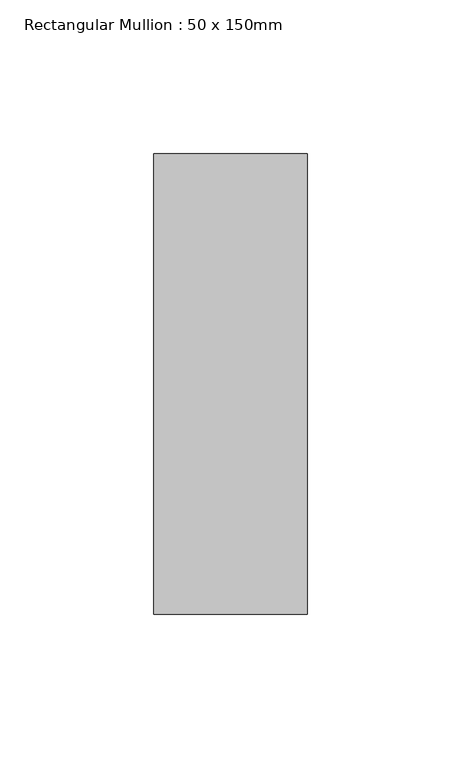
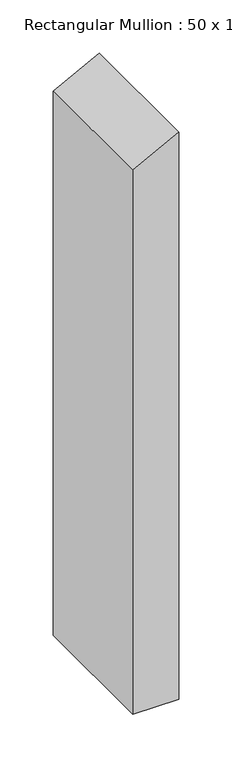
"""IFC4 building model written with IfcOpenShell, lengths in millimetres: member geometry, Rectangular Mullion : 50 x 150mm."""

from ifc_helpers import new_model, si_unit, frame, origin, place, context, project, spatial, polyline, outline, extrude, source, transform, mapped, element, save


def rectangular_mullion_50_x_150mm_71cd5d06(model_context):
    return source(origin(), model_context, "Body", "SweptSolid", [
        extrude(outline(polyline([(0.0, 0.0), (-26.0283525, -50.0), (-651.6744496, -50.0), (-651.6744496, 0.0), (0.0, 0.0)])), frame((0.0, -75.0, 0.0), z_axis=(0.0, 1.0, 0.0), x_axis=(0.0, 0.0, 1.0)), (0.0, 0.0, 1.0), 150.0),
    ])


if __name__ == "__main__":
    model = new_model("IFC4")
    model_context = context("Model", 3, world=origin())
    ifc_project = project(units=[si_unit("LENGTHUNIT", "METRE", prefix="MILLI")], contexts=[model_context])
    site = spatial("IfcSite", under=ifc_project)
    building = spatial("IfcBuilding", under=site)
    placement = place(None, origin())
    rectangular_mullion_50_x_150mm_shape = rectangular_mullion_50_x_150mm_71cd5d06(model_context)
    element("IfcMember", 1, ObjectType="Rectangular Mullion : 50 x 150mm", at=placement, inside=building, context=model_context, shape_type="MappedRepresentation", body=[
        mapped(rectangular_mullion_50_x_150mm_shape, transform((0.0, 0.0, 0.0), x_axis=(1.0, 0.0, 0.0), y_axis=(0.0, 1.0, 0.0), z_axis=(0.0, 0.0, 1.0))),
    ])
    save(model, "model.ifc")

# Revit data of these elements
# Type "Rectangular Mullion : 50 x 150mm"
#   built-in parameter 1007304 = 0.492126 (stored number, unit not read)
#   built-in parameter 1007301 = 0.082021 (stored number, unit not read)
#   built-in parameter 1007300 = 0.082021 (stored number, unit not read)
# Element 1 (IfcMember, "Rectangular Mullion : 50 x 150mm")
#   Materials on its faces: "Aluminium"
# Materials
#   "Aluminium": class "Metal", colour RGB 247 247 247, transparency 0, Description = "Aluminium 6061", Cost = 0
